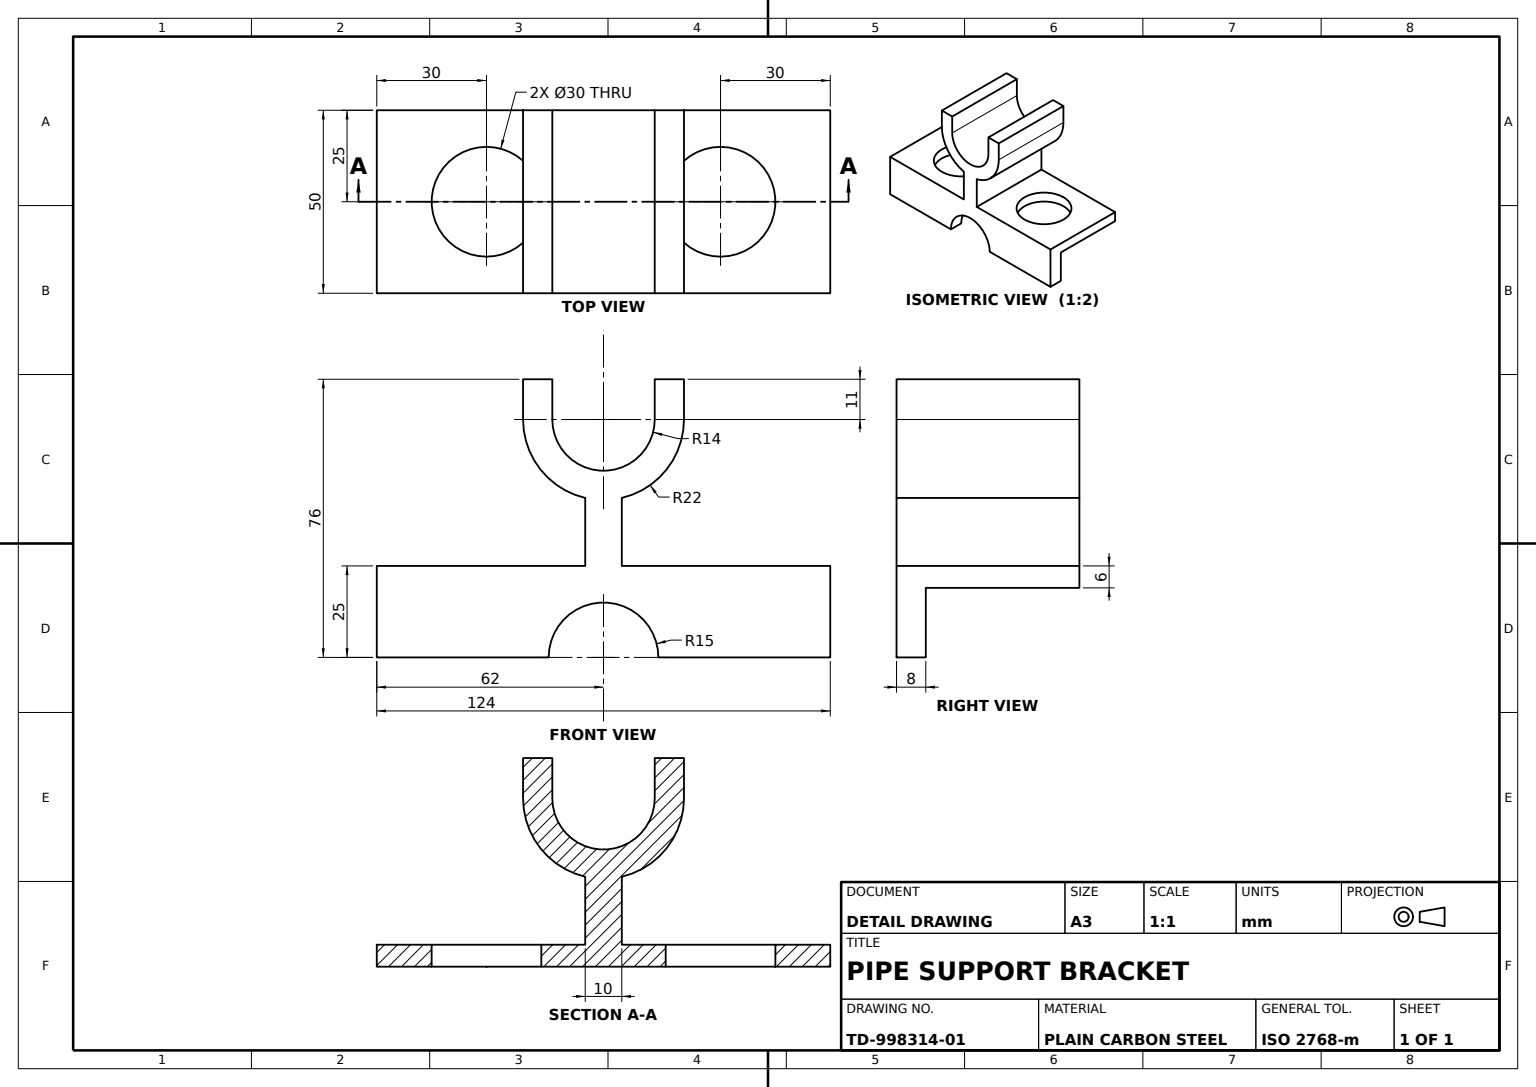
from build123d import *

# Parameters (mm, degrees)
BRACKET_BODY_DEPTH         = 25
CRADLE_SLOT_CUT_DEPTH      = 148.57032222
CRADLE_SLOT_CUT_DEPTH_BACK = 148.57032222
CRADLE_SLOT_SKETCH_W       = 42
CRADLE_SLOT_SKETCH_H       = 19
BASE_CUT_OUT_SKETCH_R      = 15
BASE_CUT_OUTS_DEPTH        = 85.083292038


with BuildPart() as part:
    # Bracket Profile Sketch → Bracket Body (new, symmetric)
    with BuildSketch(Plane.XY):
        with BuildLine():
            Line((-62, 0), (-15, 0))
            ThreePointArc((-15, 0), (0, 15), (15, 0))
            Line((15, 0), (62, 0))
            Line((62, 0), (62, 25))
            Line((62, 25), (5, 25))
            Line((5, 25), (5, 43.575714714))
            ThreePointArc((5, 43.575714714), (17.23368794, 51.325205669), (22, 65))
            Line((22, 65), (22, 76))
            Line((22, 76), (14, 76))
            Line((14, 76), (14, 65))
            ThreePointArc((14, 65), (0, 51), (-14, 65))
            Line((-14, 65), (-14, 76))
            Line((-14, 76), (-22, 76))
            Line((-22, 76), (-22, 65))
            ThreePointArc((-22, 65), (-17.23368794, 51.325205669), (-5, 43.575714714))
            Line((-5, 43.575714714), (-5, 25))
            Line((-5, 25), (-62, 25))
            Line((-62, 25), (-62, 0))
        make_face()
    extrude(amount=BRACKET_BODY_DEPTH, both=True)

    # Cradle Slot Sketch → Cradle Slot Cut (cut, two sides: drawn at the far end of the back side and taken through both)
    with BuildSketch(Plane(origin=(62, 0, 0), x_dir=(0, 0, -1), z_dir=(1, 0, 0)).offset(-CRADLE_SLOT_CUT_DEPTH_BACK)):
        with Locations((4, 9.5)):
            Rectangle(CRADLE_SLOT_SKETCH_W, CRADLE_SLOT_SKETCH_H)
    extrude(amount=CRADLE_SLOT_CUT_DEPTH + CRADLE_SLOT_CUT_DEPTH_BACK, mode=Mode.SUBTRACT)

    # Base Cut-Out Sketch → Base Cut-Outs (cut, through all)
    with BuildSketch(Plane(origin=(0, 25, 0), x_dir=(1, 0, 0), z_dir=(0, 1, 0))):
        with Locations(Location((-32, 0, 0), (0, 0, 270))):
            Circle(BASE_CUT_OUT_SKETCH_R)
        with Locations(Location((32, 0, 0), (0, 0, 270))):
            Circle(BASE_CUT_OUT_SKETCH_R)
    extrude(amount=-BASE_CUT_OUTS_DEPTH, mode=Mode.SUBTRACT)


solid = part.part
